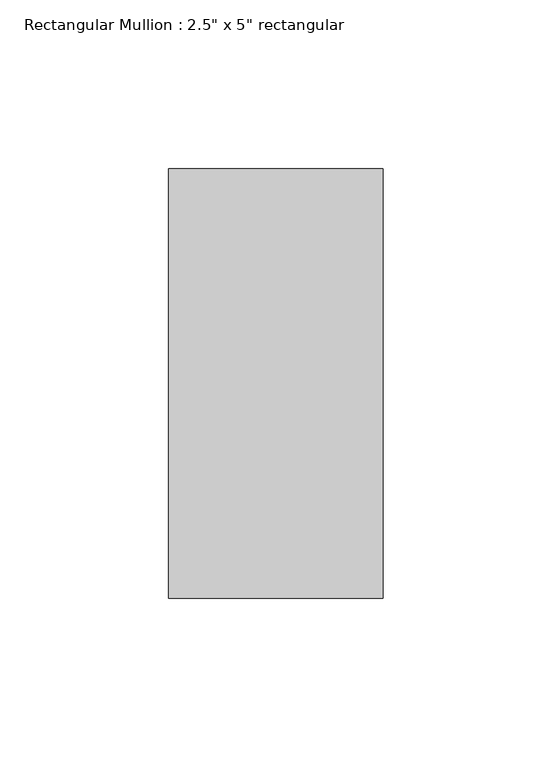
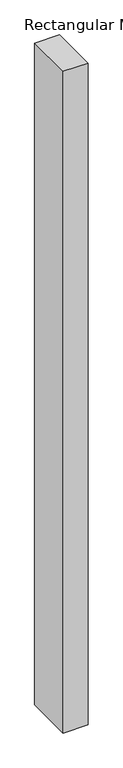
"""IFC4 building model written with IfcOpenShell, lengths in millimetres: member geometry."""

from ifc_helpers import new_model, si_unit, frame, origin, place, context, project, spatial, polyline, outline, extrude, source, transform, mapped, element, save


def member_5295ae1b(model_context):
    return source(origin(), model_context, "Body", "SweptSolid", [
        extrude(outline(polyline([(0.0, 63.5), (0.0, -63.5), (-63.5, -63.5), (-63.5, 63.5), (0.0, 63.5)])), frame((0.0, 0.0, -1798.7548712), z_axis=(0.0, 0.0, 1.0), x_axis=(1.0, 0.0, 0.0)), (0.0, 0.0, 1.0), 1798.7548712),
    ])


if __name__ == "__main__":
    model = new_model("IFC4")
    model_context = context("Model", 3, world=origin())
    ifc_project = project(units=[si_unit("LENGTHUNIT", "METRE", prefix="MILLI")], contexts=[model_context])
    site = spatial("IfcSite", under=ifc_project)
    building = spatial("IfcBuilding", under=site)
    placement = place(None, origin())
    member_shape = member_5295ae1b(model_context)
    element("IfcMember", 1, ObjectType="Rectangular Mullion : 2.5\" x 5\" rectangular", at=placement, inside=building, context=model_context, shape_type="MappedRepresentation", body=[
        mapped(member_shape, transform((0.0, 0.0, 0.0), x_axis=(1.0, 0.0, 0.0), y_axis=(0.0, 1.0, 0.0), z_axis=(0.0, 0.0, 1.0))),
    ])
    save(model, "model.ifc")

# Revit data of these elements
# Type "Rectangular Mullion : 2.5\" x 5\" rectangular"
#   built-in parameter 1007304 = 0.416667 (stored number, unit not read)
#   built-in parameter 1007301 = 0.104167 (stored number, unit not read)
#   built-in parameter 1007300 = 0.104167 (stored number, unit not read)
# Element 1 (IfcMember, "Rectangular Mullion : 2.5\" x 5\" rectangular")
#   Materials on its faces: "Aluminum"
# Materials
#   "Aluminum": class "Metal", colour RGB 247 247 247, transparency 0, Description = "Aluminum 6061", Cost = 0
